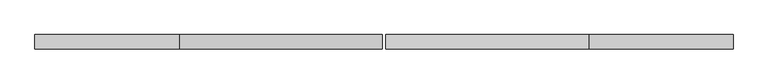
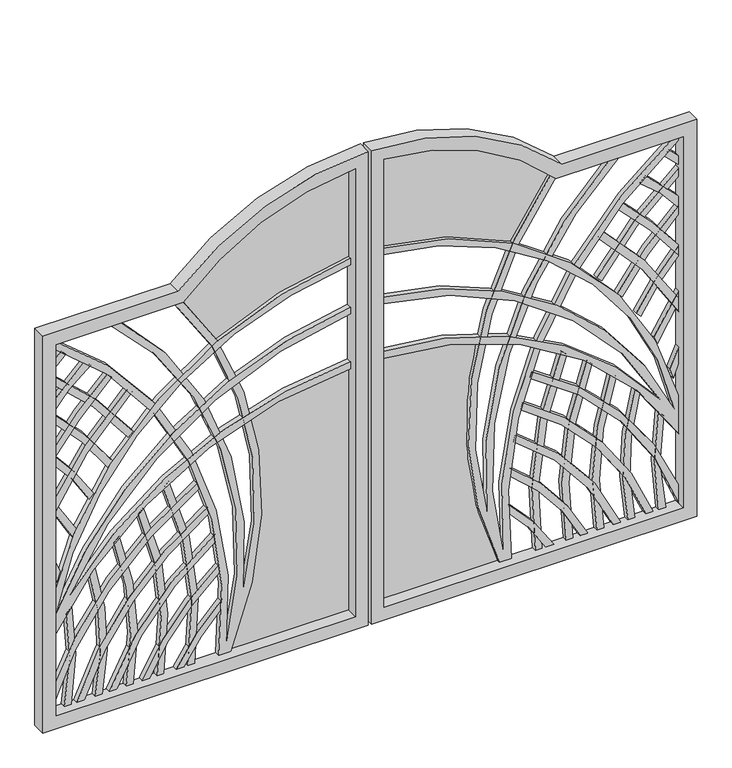
"""IFC4 building model written with IfcOpenShell, lengths in millimetres: proxy geometry."""

from ifc_helpers import new_model, si_unit, point, frame, frame_2d, origin, place, context, project, spatial, polyline, circle_curve, trimmed, segment, composite_curve, outline, extrude, source, transform, mapped, element, save


def generic_models_6bc30956(model_context):
    return source(origin(), model_context, "Body", "SweptSolid", [
        extrude(outline(composite_curve([segment(polyline([(1574.8, -714.375), (1574.8, -1222.375), (0.0, -1222.375), (0.0, 0.0), (1879.3736556, 0.0)]), True, "CONTINUOUS"), segment(trimmed(circle_curve(frame_2d((881.859553, 3.175)), 997.5191555), [point((1879.3736556, 0.0))], [point((1574.8, -714.375))], False, "CARTESIAN"), True, "CONTINUOUS")], self_intersect=False), holes=[composite_curve([segment(polyline([(1827.2147875, -47.625), (50.8, -47.625), (50.8, -1171.575), (1524.0, -1171.575), (1524.0, -692.4777911)]), True, "CONTINUOUS"), segment(trimmed(circle_curve(frame_2d((881.859553, 3.175)), 946.7191555), [point((1524.0, -692.4777911))], [point((1827.2147875, -47.625))], True, "CARTESIAN"), True, "CONTINUOUS")], self_intersect=False)]), frame((0.0, -50.8, 0.0), z_axis=(0.0, 1.0, 0.0), x_axis=(0.0, 0.0, 1.0)), (0.0, 0.0, 1.0), 50.8),
        extrude(outline(composite_curve([segment(trimmed(circle_curve(frame_2d((188.1193765, 65.6258097)), 1270.1981582), [point((1453.2587424, -47.625))], [point((475.7606767, -1171.575))], False, "CARTESIAN"), True, "CONTINUOUS"), segment(polyline([(475.7606767, -1171.575), (325.438753, -1171.575)]), True, "CONTINUOUS"), segment(trimmed(circle_curve(frame_2d((-306.470048, -9.2092819)), 1323.0278891), [point((325.438753, -1171.575))], [point((1016.0, -47.625))], True, "CARTESIAN"), True, "CONTINUOUS"), segment(polyline([(1016.0, -47.625), (1042.85139, -47.625)]), True, "CONTINUOUS"), segment(trimmed(circle_curve(frame_2d((-321.9912288, -1.7370637)), 1365.6138095), [point((1042.85139, -47.625))], [point((487.9033995, -1101.269586))], False, "CARTESIAN"), True, "CONTINUOUS"), segment(trimmed(circle_curve(frame_2d((-94.5667128, 101.7568292)), 1336.6166195), [point((487.9033995, -1101.269586))], [point((1233.6761327, -47.625))], True, "CARTESIAN"), True, "CONTINUOUS"), segment(polyline([(1233.6761327, -47.625), (1259.2332506, -47.625)]), True, "CONTINUOUS"), segment(trimmed(circle_curve(frame_2d((-94.5667128, 101.7568292)), 1362.0166195), [point((1259.2332506, -47.625))], [point((428.8390935, -1155.6753295))], False, "CARTESIAN"), True, "CONTINUOUS"), segment(trimmed(circle_curve(frame_2d((188.1193765, 65.6258097)), 1244.7981582), [point((428.8390935, -1155.6753295))], [point((1427.7550927, -47.625))], True, "CARTESIAN"), True, "CONTINUOUS"), segment(polyline([(1427.7550927, -47.625), (1453.2587424, -47.625)]), True, "CONTINUOUS")], self_intersect=False)), frame((0.0, -19.05, 0.0), z_axis=(0.0, 1.0, 0.0), x_axis=(0.0, 0.0, 1.0)), (0.0, 0.0, 1.0), 19.05),
        extrude(outline(composite_curve([segment(trimmed(circle_curve(frame_2d((625.1927136, -1831.8247988)), 1451.1947292), [point((50.8, -499.1436094))], [point((1524.0, -692.4777911))], False, "CARTESIAN"), True, "CONTINUOUS"), segment(polyline([(1524.0, -692.4777911), (1524.0, -717.8616311), (1508.2761961, -712.4096154)]), True, "CONTINUOUS"), segment(trimmed(circle_curve(frame_2d((625.2005352, -1831.8604357)), 1425.8305516), [point((1508.2761961, -712.4096154))], [point((270.5135839, -450.849962))], True, "CARTESIAN"), True, "CONTINUOUS"), segment(trimmed(circle_curve(frame_2d((428.9211986, -1911.4736244)), 1469.1883662), [point((270.5135839, -450.849962))], [point((1524.0, -932.0263955))], False, "CARTESIAN"), True, "CONTINUOUS"), segment(polyline([(1524.0, -932.0263955), (1524.0, -970.5462776)]), True, "CONTINUOUS"), segment(trimmed(circle_curve(frame_2d((434.6192112, -1905.6521568)), 1435.6787622), [point((1524.0, -970.5462776))], [point((79.5169904, -514.5820935))], True, "CARTESIAN"), True, "CONTINUOUS"), segment(trimmed(circle_curve(frame_2d((251.9754674, -2051.8469137)), 1546.9082241), [point((79.5169904, -514.5820935))], [point((1524.0, -1171.575))], False, "CARTESIAN"), True, "CONTINUOUS"), segment(polyline([(1524.0, -1171.575), (1492.986601, -1171.575)]), True, "CONTINUOUS"), segment(trimmed(circle_curve(frame_2d((251.9754674, -2051.8469137)), 1521.5082241), [point((1492.986601, -1171.575))], [point((50.8, -543.6971508))], True, "CARTESIAN"), True, "CONTINUOUS"), segment(polyline([(50.8, -543.6971508), (50.8, -499.1436094)]), True, "CONTINUOUS")], self_intersect=False)), frame((0.0, -19.05, 0.0), z_axis=(0.0, 1.0, 0.0), x_axis=(0.0, 0.0, 1.0)), (0.0, 0.0, 1.0), 19.05),
        extrude(outline(composite_curve([segment(trimmed(circle_curve(frame_2d((-321.9912288, -1.7370636)), 1251.3138095), [point((766.023996, -619.8059275))], [point((122.1545272, -1171.575))], False, "CARTESIAN"), True, "CONTINUOUS"), segment(polyline([(122.1545272, -1171.575), (50.8, -1171.575)]), True, "CONTINUOUS"), segment(trimmed(circle_curve(frame_2d((-329.3476454, 3.2021804)), 1234.7524675), [point((50.8, -1171.575))], [point((741.6413557, -611.2864))], True, "CARTESIAN"), True, "CONTINUOUS"), segment(polyline([(741.6413557, -611.2864), (766.023996, -619.8059275)]), True, "CONTINUOUS")], self_intersect=False)), frame((0.0, -19.05, 0.0), z_axis=(0.0, 1.0, 0.0), x_axis=(0.0, 0.0, 1.0)), (0.0, 0.0, 1.0), 19.05),
        extrude(outline(composite_curve([segment(trimmed(circle_curve(frame_2d((-321.9912288, -1.7370637)), 1137.0138095), [point((654.3216834, -584.5007383))], [point((50.8, -1075.9005069))], False, "CARTESIAN"), True, "CONTINUOUS"), segment(polyline([(50.8, -1075.9005069), (50.8, -1048.9772277)]), True, "CONTINUOUS"), segment(trimmed(circle_curve(frame_2d((-321.9912288, -1.7370637)), 1111.6138095), [point((50.8, -1048.9772277))], [point((628.7552213, -577.7287729))], True, "CARTESIAN"), True, "CONTINUOUS"), segment(polyline([(628.7552213, -577.7287729), (654.3216834, -584.5007383)]), True, "CONTINUOUS")], self_intersect=False)), frame((0.0, -19.05, 0.0), z_axis=(0.0, 1.0, 0.0), x_axis=(0.0, 0.0, 1.0)), (0.0, 0.0, 1.0), 19.05),
        extrude(outline(composite_curve([segment(trimmed(circle_curve(frame_2d((-321.9912288, -1.7370637)), 1022.7138095), [point((536.7182406, -557.2202617))], [point((50.8, -954.0869132))], False, "CARTESIAN"), True, "CONTINUOUS"), segment(polyline([(50.8, -954.0869132), (50.8, -926.7568118)]), True, "CONTINUOUS"), segment(trimmed(circle_curve(frame_2d((-321.9912288, -1.7370637)), 997.3138095), [point((50.8, -926.7568118))], [point((510.8571668, -550.3702604))], True, "CARTESIAN"), True, "CONTINUOUS"), segment(polyline([(510.8571668, -550.3702604), (536.7182406, -557.2202617)]), True, "CONTINUOUS")], self_intersect=False)), frame((0.0, -19.05, 0.0), z_axis=(0.0, 1.0, 0.0), x_axis=(0.0, 0.0, 1.0)), (0.0, 0.0, 1.0), 19.05),
        extrude(outline(composite_curve([segment(trimmed(circle_curve(frame_2d((-321.9912288, -1.7370637)), 908.4138095), [point((410.7722159, -538.6480277))], [point((50.8, -830.134522))], False, "CARTESIAN"), True, "CONTINUOUS"), segment(polyline([(50.8, -830.134522), (50.8, -802.1994847)]), True, "CONTINUOUS"), segment(trimmed(circle_curve(frame_2d((-321.9912288, -1.7370637)), 883.0138095), [point((50.8, -802.1994847))], [point((379.0365912, -538.6480277))], True, "CARTESIAN"), True, "CONTINUOUS"), segment(polyline([(379.0365912, -538.6480277), (410.7722159, -538.6480277)]), True, "CONTINUOUS")], self_intersect=False)), frame((0.0, -19.05, 0.0), z_axis=(0.0, 1.0, 0.0), x_axis=(0.0, 0.0, 1.0)), (0.0, 0.0, 1.0), 19.05),
        extrude(outline(composite_curve([segment(trimmed(circle_curve(frame_2d((-321.9912288, -1.7370637)), 794.1138095), [point((270.5266887, -530.4517881))], [point((50.8, -702.9099683))], False, "CARTESIAN"), True, "CONTINUOUS"), segment(polyline([(50.8, -702.9099683), (50.8, -674.0075603)]), True, "CONTINUOUS"), segment(trimmed(circle_curve(frame_2d((-321.9912288, -1.7370637)), 768.7138095), [point((50.8, -674.0075603))], [point((236.0245963, -530.4517881))], True, "CARTESIAN"), True, "CONTINUOUS"), segment(polyline([(236.0245963, -530.4517881), (270.5266887, -530.4517881)]), True, "CONTINUOUS")], self_intersect=False)), frame((0.0, -19.05, 0.0), z_axis=(0.0, 1.0, 0.0), x_axis=(0.0, 0.0, 1.0)), (0.0, 0.0, 1.0), 19.05),
        extrude(outline(composite_curve([segment(polyline([(1210.9602193, -867.4506933), (1228.939295, -885.429769)]), True, "CONTINUOUS"), segment(trimmed(circle_curve(frame_2d((188.1193765, 65.6258097)), 1409.8981582), [point((1228.939295, -885.429769))], [point((864.245824, -1171.575))], False, "CARTESIAN"), True, "CONTINUOUS"), segment(polyline([(864.245824, -1171.575), (809.5445985, -1171.575)]), True, "CONTINUOUS"), segment(trimmed(circle_curve(frame_2d((188.1193765, 65.6258097)), 1384.4981582), [point((809.5445985, -1171.575))], [point((1210.9602193, -867.4506933))], True, "CARTESIAN"), True, "CONTINUOUS")], self_intersect=False)), frame((0.0, -19.05, 0.0), z_axis=(0.0, 1.0, 0.0), x_axis=(0.0, 0.0, 1.0)), (0.0, 0.0, 1.0), 19.05),
        extrude(outline(composite_curve([segment(polyline([(1295.7670706, -944.0833092), (1313.7464656, -962.0627043)]), True, "CONTINUOUS"), segment(trimmed(circle_curve(frame_2d((298.9547736, -40.580869)), 1370.7410225), [point((1313.7464656, -962.0627043))], [point((1073.4115036, -1171.575))], False, "CARTESIAN"), True, "CONTINUOUS"), segment(polyline([(1073.4115036, -1171.575), (1034.1276953, -1171.575)]), True, "CONTINUOUS"), segment(trimmed(circle_curve(frame_2d((188.1193765, 65.6258097)), 1498.7981582), [point((1034.1276953, -1171.575))], [point((1295.7670706, -944.0833092))], True, "CARTESIAN"), True, "CONTINUOUS")], self_intersect=False)), frame((0.0, -19.05, 0.0), z_axis=(0.0, 1.0, 0.0), x_axis=(0.0, 0.0, 1.0)), (0.0, 0.0, 1.0), 19.05),
        extrude(outline(composite_curve([segment(polyline([(1371.3808408, -1023.8325474), (1393.8084123, -1046.2601189)]), True, "CONTINUOUS"), segment(trimmed(circle_curve(frame_2d((157.0059526, 65.2274597)), 1662.854462), [point((1393.8084123, -1046.2601189))], [point((1268.4935312, -1171.575))], False, "CARTESIAN"), True, "CONTINUOUS"), segment(polyline([(1268.4935312, -1171.575), (1223.2134903, -1171.575)]), True, "CONTINUOUS"), segment(trimmed(circle_curve(frame_2d((881.0604584, -680.2699964)), 598.7063586), [point((1223.2134903, -1171.575))], [point((1371.3808408, -1023.8325474))], True, "CARTESIAN"), True, "CONTINUOUS")], self_intersect=False)), frame((0.0, -19.05, 0.0), z_axis=(0.0, 1.0, 0.0), x_axis=(0.0, 0.0, 1.0)), (0.0, 0.0, 1.0), 19.05),
        extrude(outline(composite_curve([segment(polyline([(1448.1437026, -1116.942791), (1466.2607278, -1135.0598162)]), True, "CONTINUOUS"), segment(trimmed(circle_curve(frame_2d((2369.5144168, -2074.828689)), 1303.469509), [point((1466.2607278, -1135.0598162))], [point((1429.745544, -1171.575))], True, "CARTESIAN"), True, "CONTINUOUS"), segment(polyline([(1429.745544, -1171.575), (1393.6228205, -1171.575)]), True, "CONTINUOUS"), segment(trimmed(circle_curve(frame_2d((2581.8039176, -2302.8138821)), 1640.5717686), [point((1393.6228205, -1171.575))], [point((1448.1437026, -1116.942791))], False, "CARTESIAN"), True, "CONTINUOUS")], self_intersect=False)), frame((0.0, -19.05, 0.0), z_axis=(0.0, 1.0, 0.0), x_axis=(0.0, 0.0, 1.0)), (0.0, 0.0, 1.0), 19.05),
        extrude(outline(composite_curve([segment(polyline([(50.8, -1123.3836365), (50.8, -1096.2682984)]), True, "CONTINUOUS"), segment(trimmed(circle_curve(frame_2d((249.227799, -2294.693819)), 1214.741668), [point((50.8, -1096.2682984))], [point((439.2593722, -1094.9082877))], False, "CARTESIAN"), True, "CONTINUOUS"), segment(polyline([(439.2593722, -1094.9082877), (417.7529701, -1116.4146899)]), True, "CONTINUOUS"), segment(trimmed(circle_curve(frame_2d((251.9754674, -2051.8469137)), 950.0082241), [point((417.7529701, -1116.4146899))], [point((50.8, -1123.3836365))], True, "CARTESIAN"), True, "CONTINUOUS")], self_intersect=False)), frame((0.0, -19.05, 0.0), z_axis=(0.0, 1.0, 0.0), x_axis=(0.0, 0.0, 1.0)), (0.0, 0.0, 1.0), 19.05),
        extrude(outline(composite_curve([segment(polyline([(50.8, -1006.7247069), (50.8, -980.869582)]), True, "CONTINUOUS"), segment(trimmed(circle_curve(frame_2d((251.9754674, -2051.8469137)), 1089.7082241), [point((50.8, -980.869582))], [point((559.4182819, -1006.4078053))], False, "CARTESIAN"), True, "CONTINUOUS"), segment(polyline([(559.4182819, -1006.4078053), (538.8861292, -1026.939958)]), True, "CONTINUOUS"), segment(trimmed(circle_curve(frame_2d((251.9754674, -2051.8469137)), 1064.3082241), [point((538.8861292, -1026.939958))], [point((50.8, -1006.7247069))], True, "CARTESIAN"), True, "CONTINUOUS")], self_intersect=False)), frame((0.0, -19.05, 0.0), z_axis=(0.0, 1.0, 0.0), x_axis=(0.0, 0.0, 1.0)), (0.0, 0.0, 1.0), 19.05),
        extrude(outline(composite_curve([segment(polyline([(50.8, -890.30598), (50.8, -864.7646777)]), True, "CONTINUOUS"), segment(trimmed(circle_curve(frame_2d((251.9754674, -2051.8469137)), 1204.0082241), [point((50.8, -864.7646777))], [point((656.0575932, -917.6716895))], False, "CARTESIAN"), True, "CONTINUOUS"), segment(polyline([(656.0575932, -917.6716895), (636.1282841, -937.6009986)]), True, "CONTINUOUS"), segment(trimmed(circle_curve(frame_2d((249.671635, -2074.7397377)), 1201.0134277), [point((636.1282841, -937.6009986))], [point((50.8, -890.30598))], True, "CARTESIAN"), True, "CONTINUOUS")], self_intersect=False)), frame((0.0, -19.05, 0.0), z_axis=(0.0, 1.0, 0.0), x_axis=(0.0, 0.0, 1.0)), (0.0, 0.0, 1.0), 19.05),
        extrude(outline(composite_curve([segment(polyline([(50.8, -774.6859578), (50.8, -748.9789216)]), True, "CONTINUOUS"), segment(trimmed(circle_curve(frame_2d((251.9754674, -2051.8469137)), 1318.3082241), [point((50.8, -748.9789216))], [point((737.9350335, -826.3756274))], False, "CARTESIAN"), True, "CONTINUOUS"), segment(polyline([(737.9350335, -826.3756274), (718.3335001, -845.9771607)]), True, "CONTINUOUS"), segment(trimmed(circle_curve(frame_2d((251.9754674, -2051.8469137)), 1292.9082241), [point((718.3335001, -845.9771607))], [point((50.8, -774.6859578))], True, "CARTESIAN"), True, "CONTINUOUS")], self_intersect=False)), frame((0.0, -19.05, 0.0), z_axis=(0.0, 1.0, 0.0), x_axis=(0.0, 0.0, 1.0)), (0.0, 0.0, 1.0), 19.05),
        extrude(outline(composite_curve([segment(polyline([(50.8, -659.0930168), (50.8, -633.4341547)]), True, "CONTINUOUS"), segment(trimmed(circle_curve(frame_2d((251.9754674, -2051.8469137)), 1432.6082241), [point((50.8, -633.4341547))], [point((808.380048, -731.7028813))], False, "CARTESIAN"), True, "CONTINUOUS"), segment(polyline([(808.380048, -731.7028813), (788.9599222, -751.1230071)]), True, "CONTINUOUS"), segment(trimmed(circle_curve(frame_2d((251.9754674, -2051.8469137)), 1407.2082241), [point((788.9599222, -751.1230071))], [point((50.8, -659.0930168))], True, "CARTESIAN"), True, "CONTINUOUS")], self_intersect=False)), frame((0.0, -19.05, 0.0), z_axis=(0.0, 1.0, 0.0), x_axis=(0.0, 0.0, 1.0)), (0.0, 0.0, 1.0), 19.05),
        extrude(outline(polyline([(553.3842288, -1150.9205103), (593.450224, -1138.1641492), (672.1451492, -1171.575), (609.2386529, -1171.575), (553.3842288, -1150.9205103)])), frame((0.0, -19.05, 0.0), z_axis=(0.0, 1.0, 0.0), x_axis=(0.0, 0.0, 1.0)), (0.0, 0.0, 1.0), 19.05),
        extrude(outline(composite_curve([segment(trimmed(circle_curve(frame_2d((251.9754673, -2051.8469137)), 1064.3082241), [point((850.2006371, -1171.575))], [point((711.3700205, -1091.7903318))], True, "CARTESIAN"), True, "CONTINUOUS"), segment(polyline([(711.3700205, -1091.7903318), (740.9012216, -1077.980588)]), True, "CONTINUOUS"), segment(trimmed(circle_curve(frame_2d((251.9754674, -2051.8469137)), 1089.7082241), [point((740.9012216, -1077.980588))], [point((894.3035545, -1171.575))], False, "CARTESIAN"), True, "CONTINUOUS"), segment(polyline([(894.3035545, -1171.575), (850.2006371, -1171.575)]), True, "CONTINUOUS")], self_intersect=False)), frame((0.0, -19.05, 0.0), z_axis=(0.0, 1.0, 0.0), x_axis=(0.0, 0.0, 1.0)), (0.0, 0.0, 1.0), 19.05),
        extrude(outline(composite_curve([segment(trimmed(circle_curve(frame_2d((436.5150762, -1780.3292563)), 853.0665783), [point((1034.1276953, -1171.575))], [point((842.2813497, -1029.9451424))], True, "CARTESIAN"), True, "CONTINUOUS"), segment(polyline([(842.2813497, -1029.9451424), (859.7363544, -1012.4901377)]), True, "CONTINUOUS"), segment(trimmed(circle_curve(frame_2d((251.9754673, -2051.8469137)), 1204.0082241), [point((859.7363544, -1012.4901377))], [point((1073.4115036, -1171.575))], False, "CARTESIAN"), True, "CONTINUOUS"), segment(polyline([(1073.4115036, -1171.575), (1034.1276953, -1171.575)]), True, "CONTINUOUS")], self_intersect=False)), frame((0.0, -19.05, 0.0), z_axis=(0.0, 1.0, 0.0), x_axis=(0.0, 0.0, 1.0)), (0.0, 0.0, 1.0), 19.05),
        extrude(outline(composite_curve([segment(polyline([(943.9740273, -959.7161207), (962.3717805, -941.3183675)]), True, "CONTINUOUS"), segment(trimmed(circle_curve(frame_2d((251.9754673, -2051.8469138)), 1318.3082242), [point((962.3717805, -941.3183675))], [point((1233.3306179, -1171.575))], False, "CARTESIAN"), True, "CONTINUOUS"), segment(polyline([(1233.3306179, -1171.575), (1198.9353576, -1171.575)]), True, "CONTINUOUS"), segment(trimmed(circle_curve(frame_2d((251.9754673, -2051.8469138)), 1292.9082241), [point((1198.9353576, -1171.575))], [point((943.9740273, -959.7161207))], True, "CARTESIAN"), True, "CONTINUOUS")], self_intersect=False)), frame((0.0, -19.05, 0.0), z_axis=(0.0, 1.0, 0.0), x_axis=(0.0, 0.0, 1.0)), (0.0, 0.0, 1.0), 19.05),
        extrude(outline(composite_curve([segment(polyline([(1035.0267606, -882.6310833), (1053.3289179, -864.3289261)]), True, "CONTINUOUS"), segment(trimmed(circle_curve(frame_2d((251.9754673, -2051.8469137)), 1432.6082241), [point((1053.3289179, -864.3289261))], [point((1382.2354736, -1171.575))], False, "CARTESIAN"), True, "CONTINUOUS"), segment(polyline([(1382.2354736, -1171.575), (1349.8626855, -1171.575)]), True, "CONTINUOUS"), segment(trimmed(circle_curve(frame_2d((251.9754674, -2051.8469137)), 1407.2082241), [point((1349.8626855, -1171.575))], [point((1035.0267606, -882.6310833))], True, "CARTESIAN"), True, "CONTINUOUS")], self_intersect=False)), frame((0.0, -19.05, 0.0), z_axis=(0.0, 1.0, 0.0), x_axis=(0.0, 0.0, 1.0)), (0.0, 0.0, 1.0), 19.05),
        extrude(outline(composite_curve([segment(trimmed(circle_curve(frame_2d((881.859553, 3.175)), 946.7191555), [point((1827.2147875, -47.625))], [point((1524.0, -692.4777911))], False, "CARTESIAN"), True, "CONTINUOUS"), segment(trimmed(circle_curve(frame_2d((625.1927137, -1831.8247988)), 1451.1947292), [point((1524.0, -692.4777911))], [point((1300.6036994, -547.3847876))], True, "CARTESIAN"), True, "CONTINUOUS"), segment(trimmed(circle_curve(frame_2d((188.1193765, 65.6258097)), 1270.1981582), [point((1300.6036994, -547.3847876))], [point((1453.2587424, -47.625))], True, "CARTESIAN"), True, "CONTINUOUS"), segment(polyline([(1453.2587424, -47.625), (1827.2147875, -47.625)]), True, "CONTINUOUS")], self_intersect=False)), frame((0.0, -6.35, 0.0), z_axis=(0.0, 1.0, 0.0), x_axis=(0.0, 0.0, 1.0)), (0.0, 0.0, 1.0), 6.35),
        extrude(outline(composite_curve([segment(trimmed(circle_curve(frame_2d((-306.470048, -9.2092819)), 1323.0278891), [point((1016.0, -47.625))], [point((951.8602911, -417.8748577))], False, "CARTESIAN"), True, "CONTINUOUS"), segment(trimmed(circle_curve(frame_2d((625.1927136, -1831.8247988)), 1451.1947292), [point((951.8602911, -417.8748577))], [point((50.8, -499.1436094))], True, "CARTESIAN"), True, "CONTINUOUS"), segment(polyline([(50.8, -499.1436094), (50.8, -47.625), (1016.0, -47.625)]), True, "CONTINUOUS")], self_intersect=False)), frame((0.0, -6.35, 0.0), z_axis=(0.0, 1.0, 0.0), x_axis=(0.0, 0.0, 1.0)), (0.0, 0.0, 1.0), 6.35),
        extrude(outline(composite_curve([segment(trimmed(circle_curve(frame_2d((881.859553, 9.525)), 997.5191555), [point((1574.8, 727.075))], [point((1879.3736556, 12.7))], False, "CARTESIAN"), True, "CONTINUOUS"), segment(polyline([(1879.3736556, 12.7), (0.0, 12.7), (0.0, 1235.075), (1574.8, 1235.075), (1574.8, 727.075)]), True, "CONTINUOUS")], self_intersect=False), holes=[composite_curve([segment(trimmed(circle_curve(frame_2d((881.859553, 9.525)), 946.7191555), [point((1827.2147875, 60.325))], [point((1524.0, 705.1777911))], True, "CARTESIAN"), True, "CONTINUOUS"), segment(polyline([(1524.0, 705.1777911), (1524.0, 1184.275), (50.8, 1184.275), (50.8, 60.325), (1827.2147875, 60.325)]), True, "CONTINUOUS")], self_intersect=False)]), frame((0.0, -50.8, 0.0), z_axis=(0.0, 1.0, 0.0), x_axis=(0.0, 0.0, 1.0)), (0.0, 0.0, 1.0), 50.8),
        extrude(outline(composite_curve([segment(polyline([(1453.2587424, 60.325), (1427.7550927, 60.325)]), True, "CONTINUOUS"), segment(trimmed(circle_curve(frame_2d((188.1193765, -52.9258097)), 1244.7981582), [point((1427.7550927, 60.325))], [point((428.8390935, 1168.3753295))], True, "CARTESIAN"), True, "CONTINUOUS"), segment(trimmed(circle_curve(frame_2d((-94.5667128, -89.0568292)), 1362.0166195), [point((428.8390935, 1168.3753295))], [point((1259.2332506, 60.325))], False, "CARTESIAN"), True, "CONTINUOUS"), segment(polyline([(1259.2332506, 60.325), (1233.6761327, 60.325)]), True, "CONTINUOUS"), segment(trimmed(circle_curve(frame_2d((-94.5667128, -89.0568292)), 1336.6166195), [point((1233.6761327, 60.325))], [point((487.9033995, 1113.969586))], True, "CARTESIAN"), True, "CONTINUOUS"), segment(trimmed(circle_curve(frame_2d((-321.9912288, 14.4370637)), 1365.6138095), [point((487.9033995, 1113.969586))], [point((1042.85139, 60.325))], False, "CARTESIAN"), True, "CONTINUOUS"), segment(polyline([(1042.85139, 60.325), (1016.0, 60.325)]), True, "CONTINUOUS"), segment(trimmed(circle_curve(frame_2d((-306.470048, 21.9092819)), 1323.0278891), [point((1016.0, 60.325))], [point((325.438753, 1184.275))], True, "CARTESIAN"), True, "CONTINUOUS"), segment(polyline([(325.438753, 1184.275), (475.7606767, 1184.275)]), True, "CONTINUOUS"), segment(trimmed(circle_curve(frame_2d((188.1193765, -52.9258097)), 1270.1981582), [point((475.7606767, 1184.275))], [point((1453.2587424, 60.325))], False, "CARTESIAN"), True, "CONTINUOUS")], self_intersect=False)), frame((0.0, -19.05, 0.0), z_axis=(0.0, 1.0, 0.0), x_axis=(0.0, 0.0, 1.0)), (0.0, 0.0, 1.0), 19.05),
        extrude(outline(composite_curve([segment(polyline([(50.8, 511.8436094), (50.8, 556.3971508)]), True, "CONTINUOUS"), segment(trimmed(circle_curve(frame_2d((251.9754674, 2064.5469137)), 1521.5082241), [point((50.8, 556.3971508))], [point((1492.986601, 1184.275))], True, "CARTESIAN"), True, "CONTINUOUS"), segment(polyline([(1492.986601, 1184.275), (1524.0, 1184.275)]), True, "CONTINUOUS"), segment(trimmed(circle_curve(frame_2d((251.9754674, 2064.5469137)), 1546.9082241), [point((1524.0, 1184.275))], [point((79.5169904, 527.2820935))], False, "CARTESIAN"), True, "CONTINUOUS"), segment(trimmed(circle_curve(frame_2d((434.6192112, 1918.3521568)), 1435.6787622), [point((79.5169904, 527.2820935))], [point((1524.0, 983.2462776))], True, "CARTESIAN"), True, "CONTINUOUS"), segment(polyline([(1524.0, 983.2462776), (1524.0, 944.7263955)]), True, "CONTINUOUS"), segment(trimmed(circle_curve(frame_2d((428.9211986, 1924.1736244)), 1469.1883662), [point((1524.0, 944.7263955))], [point((270.5135839, 463.549962))], False, "CARTESIAN"), True, "CONTINUOUS"), segment(trimmed(circle_curve(frame_2d((625.2005352, 1844.5604357)), 1425.8305516), [point((270.5135839, 463.549962))], [point((1508.2761961, 725.1096154))], True, "CARTESIAN"), True, "CONTINUOUS"), segment(polyline([(1508.2761961, 725.1096154), (1524.0, 730.5616311), (1524.0, 705.1777911)]), True, "CONTINUOUS"), segment(trimmed(circle_curve(frame_2d((625.1927136, 1844.5247988)), 1451.1947292), [point((1524.0, 705.1777911))], [point((50.8, 511.8436094))], False, "CARTESIAN"), True, "CONTINUOUS")], self_intersect=False)), frame((0.0, -19.05, 0.0), z_axis=(0.0, 1.0, 0.0), x_axis=(0.0, 0.0, 1.0)), (0.0, 0.0, 1.0), 19.05),
        extrude(outline(composite_curve([segment(polyline([(766.023996, 632.5059275), (741.6413557, 623.9864)]), True, "CONTINUOUS"), segment(trimmed(circle_curve(frame_2d((-329.3476454, 9.4978196)), 1234.7524675), [point((741.6413557, 623.9864))], [point((50.8, 1184.275))], True, "CARTESIAN"), True, "CONTINUOUS"), segment(polyline([(50.8, 1184.275), (122.1545272, 1184.275)]), True, "CONTINUOUS"), segment(trimmed(circle_curve(frame_2d((-321.9912288, 14.4370636)), 1251.3138095), [point((122.1545272, 1184.275))], [point((766.023996, 632.5059275))], False, "CARTESIAN"), True, "CONTINUOUS")], self_intersect=False)), frame((0.0, -19.05, 0.0), z_axis=(0.0, 1.0, 0.0), x_axis=(0.0, 0.0, 1.0)), (0.0, 0.0, 1.0), 19.05),
        extrude(outline(composite_curve([segment(polyline([(654.3216834, 597.2007383), (628.7552213, 590.4287729)]), True, "CONTINUOUS"), segment(trimmed(circle_curve(frame_2d((-321.9912288, 14.4370637)), 1111.6138095), [point((628.7552213, 590.4287729))], [point((50.8, 1061.6772277))], True, "CARTESIAN"), True, "CONTINUOUS"), segment(polyline([(50.8, 1061.6772277), (50.8, 1088.6005069)]), True, "CONTINUOUS"), segment(trimmed(circle_curve(frame_2d((-321.9912288, 14.4370637)), 1137.0138095), [point((50.8, 1088.6005069))], [point((654.3216834, 597.2007383))], False, "CARTESIAN"), True, "CONTINUOUS")], self_intersect=False)), frame((0.0, -19.05, 0.0), z_axis=(0.0, 1.0, 0.0), x_axis=(0.0, 0.0, 1.0)), (0.0, 0.0, 1.0), 19.05),
        extrude(outline(composite_curve([segment(polyline([(536.7182406, 569.9202617), (510.8571668, 563.0702604)]), True, "CONTINUOUS"), segment(trimmed(circle_curve(frame_2d((-321.9912288, 14.4370637)), 997.3138095), [point((510.8571668, 563.0702604))], [point((50.8, 939.4568118))], True, "CARTESIAN"), True, "CONTINUOUS"), segment(polyline([(50.8, 939.4568118), (50.8, 966.7869132)]), True, "CONTINUOUS"), segment(trimmed(circle_curve(frame_2d((-321.9912288, 14.4370637)), 1022.7138095), [point((50.8, 966.7869132))], [point((536.7182406, 569.9202617))], False, "CARTESIAN"), True, "CONTINUOUS")], self_intersect=False)), frame((0.0, -19.05, 0.0), z_axis=(0.0, 1.0, 0.0), x_axis=(0.0, 0.0, 1.0)), (0.0, 0.0, 1.0), 19.05),
        extrude(outline(composite_curve([segment(polyline([(410.7722159, 551.3480277), (379.0365912, 551.3480277)]), True, "CONTINUOUS"), segment(trimmed(circle_curve(frame_2d((-321.9912288, 14.4370637)), 883.0138095), [point((379.0365912, 551.3480277))], [point((50.8, 814.8994847))], True, "CARTESIAN"), True, "CONTINUOUS"), segment(polyline([(50.8, 814.8994847), (50.8, 842.834522)]), True, "CONTINUOUS"), segment(trimmed(circle_curve(frame_2d((-321.9912288, 14.4370637)), 908.4138095), [point((50.8, 842.834522))], [point((410.7722159, 551.3480277))], False, "CARTESIAN"), True, "CONTINUOUS")], self_intersect=False)), frame((0.0, -19.05, 0.0), z_axis=(0.0, 1.0, 0.0), x_axis=(0.0, 0.0, 1.0)), (0.0, 0.0, 1.0), 19.05),
        extrude(outline(composite_curve([segment(polyline([(270.5266887, 543.1517881), (236.0245963, 543.1517881)]), True, "CONTINUOUS"), segment(trimmed(circle_curve(frame_2d((-321.9912288, 14.4370637)), 768.7138095), [point((236.0245963, 543.1517881))], [point((50.8, 686.7075603))], True, "CARTESIAN"), True, "CONTINUOUS"), segment(polyline([(50.8, 686.7075603), (50.8, 715.6099683)]), True, "CONTINUOUS"), segment(trimmed(circle_curve(frame_2d((-321.9912288, 14.4370637)), 794.1138095), [point((50.8, 715.6099683))], [point((270.5266887, 543.1517881))], False, "CARTESIAN"), True, "CONTINUOUS")], self_intersect=False)), frame((0.0, -19.05, 0.0), z_axis=(0.0, 1.0, 0.0), x_axis=(0.0, 0.0, 1.0)), (0.0, 0.0, 1.0), 19.05),
        extrude(outline(composite_curve([segment(trimmed(circle_curve(frame_2d((188.1193765, -52.9258097)), 1384.4981582), [point((1210.9602193, 880.1506933))], [point((809.5445985, 1184.275))], True, "CARTESIAN"), True, "CONTINUOUS"), segment(polyline([(809.5445985, 1184.275), (864.245824, 1184.275)]), True, "CONTINUOUS"), segment(trimmed(circle_curve(frame_2d((188.1193765, -52.9258097)), 1409.8981582), [point((864.245824, 1184.275))], [point((1228.939295, 898.129769))], False, "CARTESIAN"), True, "CONTINUOUS"), segment(polyline([(1228.939295, 898.129769), (1210.9602193, 880.1506933)]), True, "CONTINUOUS")], self_intersect=False)), frame((0.0, -19.05, 0.0), z_axis=(0.0, 1.0, 0.0), x_axis=(0.0, 0.0, 1.0)), (0.0, 0.0, 1.0), 19.05),
        extrude(outline(composite_curve([segment(trimmed(circle_curve(frame_2d((188.1193765, -52.9258097)), 1498.7981582), [point((1295.7670706, 956.7833092))], [point((1034.1276953, 1184.275))], True, "CARTESIAN"), True, "CONTINUOUS"), segment(polyline([(1034.1276953, 1184.275), (1073.4115036, 1184.275)]), True, "CONTINUOUS"), segment(trimmed(circle_curve(frame_2d((298.9547736, 53.280869)), 1370.7410225), [point((1073.4115036, 1184.275))], [point((1313.7464656, 974.7627043))], False, "CARTESIAN"), True, "CONTINUOUS"), segment(polyline([(1313.7464656, 974.7627043), (1295.7670706, 956.7833092)]), True, "CONTINUOUS")], self_intersect=False)), frame((0.0, -19.05, 0.0), z_axis=(0.0, 1.0, 0.0), x_axis=(0.0, 0.0, 1.0)), (0.0, 0.0, 1.0), 19.05),
        extrude(outline(composite_curve([segment(trimmed(circle_curve(frame_2d((881.0604584, 692.9699964)), 598.7063586), [point((1371.3808408, 1036.5325474))], [point((1223.2134903, 1184.275))], True, "CARTESIAN"), True, "CONTINUOUS"), segment(polyline([(1223.2134903, 1184.275), (1268.4935312, 1184.275)]), True, "CONTINUOUS"), segment(trimmed(circle_curve(frame_2d((157.0059526, -52.5274597)), 1662.854462), [point((1268.4935312, 1184.275))], [point((1393.8084123, 1058.9601189))], False, "CARTESIAN"), True, "CONTINUOUS"), segment(polyline([(1393.8084123, 1058.9601189), (1371.3808408, 1036.5325474)]), True, "CONTINUOUS")], self_intersect=False)), frame((0.0, -19.05, 0.0), z_axis=(0.0, 1.0, 0.0), x_axis=(0.0, 0.0, 1.0)), (0.0, 0.0, 1.0), 19.05),
        extrude(outline(composite_curve([segment(trimmed(circle_curve(frame_2d((2581.8039176, 2315.5138821)), 1640.5717686), [point((1448.1437026, 1129.642791))], [point((1393.6228205, 1184.275))], False, "CARTESIAN"), True, "CONTINUOUS"), segment(polyline([(1393.6228205, 1184.275), (1429.745544, 1184.275)]), True, "CONTINUOUS"), segment(trimmed(circle_curve(frame_2d((2369.5144168, 2087.528689)), 1303.469509), [point((1429.745544, 1184.275))], [point((1466.2607278, 1147.7598162))], True, "CARTESIAN"), True, "CONTINUOUS"), segment(polyline([(1466.2607278, 1147.7598162), (1448.1437026, 1129.642791)]), True, "CONTINUOUS")], self_intersect=False)), frame((0.0, -19.05, 0.0), z_axis=(0.0, 1.0, 0.0), x_axis=(0.0, 0.0, 1.0)), (0.0, 0.0, 1.0), 19.05),
        extrude(outline(composite_curve([segment(trimmed(circle_curve(frame_2d((251.9754674, 2064.5469137)), 950.0082241), [point((50.8, 1136.0836365))], [point((417.7529701, 1129.1146899))], True, "CARTESIAN"), True, "CONTINUOUS"), segment(polyline([(417.7529701, 1129.1146899), (439.2593722, 1107.6082877)]), True, "CONTINUOUS"), segment(trimmed(circle_curve(frame_2d((249.227799, 2307.393819)), 1214.741668), [point((439.2593722, 1107.6082877))], [point((50.8, 1108.9682984))], False, "CARTESIAN"), True, "CONTINUOUS"), segment(polyline([(50.8, 1108.9682984), (50.8, 1136.0836365)]), True, "CONTINUOUS")], self_intersect=False)), frame((0.0, -19.05, 0.0), z_axis=(0.0, 1.0, 0.0), x_axis=(0.0, 0.0, 1.0)), (0.0, 0.0, 1.0), 19.05),
        extrude(outline(composite_curve([segment(trimmed(circle_curve(frame_2d((251.9754674, 2064.5469137)), 1064.3082241), [point((50.8, 1019.4247069))], [point((538.8861292, 1039.639958))], True, "CARTESIAN"), True, "CONTINUOUS"), segment(polyline([(538.8861292, 1039.639958), (559.4182819, 1019.1078053)]), True, "CONTINUOUS"), segment(trimmed(circle_curve(frame_2d((251.9754674, 2064.5469137)), 1089.7082241), [point((559.4182819, 1019.1078053))], [point((50.8, 993.569582))], False, "CARTESIAN"), True, "CONTINUOUS"), segment(polyline([(50.8, 993.569582), (50.8, 1019.4247069)]), True, "CONTINUOUS")], self_intersect=False)), frame((0.0, -19.05, 0.0), z_axis=(0.0, 1.0, 0.0), x_axis=(0.0, 0.0, 1.0)), (0.0, 0.0, 1.0), 19.05),
        extrude(outline(composite_curve([segment(trimmed(circle_curve(frame_2d((249.671635, 2087.4397377)), 1201.0134277), [point((50.8, 903.00598))], [point((636.1282841, 950.3009986))], True, "CARTESIAN"), True, "CONTINUOUS"), segment(polyline([(636.1282841, 950.3009986), (656.0575932, 930.3716895)]), True, "CONTINUOUS"), segment(trimmed(circle_curve(frame_2d((251.9754674, 2064.5469137)), 1204.0082241), [point((656.0575932, 930.3716895))], [point((50.8, 877.4646777))], False, "CARTESIAN"), True, "CONTINUOUS"), segment(polyline([(50.8, 877.4646777), (50.8, 903.00598)]), True, "CONTINUOUS")], self_intersect=False)), frame((0.0, -19.05, 0.0), z_axis=(0.0, 1.0, 0.0), x_axis=(0.0, 0.0, 1.0)), (0.0, 0.0, 1.0), 19.05),
        extrude(outline(composite_curve([segment(trimmed(circle_curve(frame_2d((251.9754674, 2064.5469137)), 1292.9082241), [point((50.8, 787.3859578))], [point((718.3335001, 858.6771607))], True, "CARTESIAN"), True, "CONTINUOUS"), segment(polyline([(718.3335001, 858.6771607), (737.9350335, 839.0756274)]), True, "CONTINUOUS"), segment(trimmed(circle_curve(frame_2d((251.9754674, 2064.5469137)), 1318.3082241), [point((737.9350335, 839.0756274))], [point((50.8, 761.6789216))], False, "CARTESIAN"), True, "CONTINUOUS"), segment(polyline([(50.8, 761.6789216), (50.8, 787.3859578)]), True, "CONTINUOUS")], self_intersect=False)), frame((0.0, -19.05, 0.0), z_axis=(0.0, 1.0, 0.0), x_axis=(0.0, 0.0, 1.0)), (0.0, 0.0, 1.0), 19.05),
        extrude(outline(composite_curve([segment(trimmed(circle_curve(frame_2d((251.9754674, 2064.5469137)), 1407.2082241), [point((50.8, 671.7930168))], [point((788.9599222, 763.8230071))], True, "CARTESIAN"), True, "CONTINUOUS"), segment(polyline([(788.9599222, 763.8230071), (808.380048, 744.4028813)]), True, "CONTINUOUS"), segment(trimmed(circle_curve(frame_2d((251.9754674, 2064.5469137)), 1432.6082241), [point((808.380048, 744.4028813))], [point((50.8, 646.1341547))], False, "CARTESIAN"), True, "CONTINUOUS"), segment(polyline([(50.8, 646.1341547), (50.8, 671.7930168)]), True, "CONTINUOUS")], self_intersect=False)), frame((0.0, -19.05, 0.0), z_axis=(0.0, 1.0, 0.0), x_axis=(0.0, 0.0, 1.0)), (0.0, 0.0, 1.0), 19.05),
        extrude(outline(polyline([(553.3842288, 1163.6205103), (609.2386529, 1184.275), (672.1451492, 1184.275), (593.450224, 1150.8641492), (553.3842288, 1163.6205103)])), frame((0.0, -19.05, 0.0), z_axis=(0.0, 1.0, 0.0), x_axis=(0.0, 0.0, 1.0)), (0.0, 0.0, 1.0), 19.05),
        extrude(outline(composite_curve([segment(polyline([(850.2006371, 1184.275), (894.3035545, 1184.275)]), True, "CONTINUOUS"), segment(trimmed(circle_curve(frame_2d((251.9754674, 2064.5469137)), 1089.7082241), [point((894.3035545, 1184.275))], [point((740.9012216, 1090.680588))], False, "CARTESIAN"), True, "CONTINUOUS"), segment(polyline([(740.9012216, 1090.680588), (711.3700205, 1104.4903318)]), True, "CONTINUOUS"), segment(trimmed(circle_curve(frame_2d((251.9754673, 2064.5469137)), 1064.3082241), [point((711.3700205, 1104.4903318))], [point((850.2006371, 1184.275))], True, "CARTESIAN"), True, "CONTINUOUS")], self_intersect=False)), frame((0.0, -19.05, 0.0), z_axis=(0.0, 1.0, 0.0), x_axis=(0.0, 0.0, 1.0)), (0.0, 0.0, 1.0), 19.05),
        extrude(outline(composite_curve([segment(polyline([(1034.1276953, 1184.275), (1073.4115036, 1184.275)]), True, "CONTINUOUS"), segment(trimmed(circle_curve(frame_2d((251.9754673, 2064.5469137)), 1204.0082241), [point((1073.4115036, 1184.275))], [point((859.7363544, 1025.1901377))], False, "CARTESIAN"), True, "CONTINUOUS"), segment(polyline([(859.7363544, 1025.1901377), (842.2813497, 1042.6451424)]), True, "CONTINUOUS"), segment(trimmed(circle_curve(frame_2d((436.5150762, 1793.0292563)), 853.0665783), [point((842.2813497, 1042.6451424))], [point((1034.1276953, 1184.275))], True, "CARTESIAN"), True, "CONTINUOUS")], self_intersect=False)), frame((0.0, -19.05, 0.0), z_axis=(0.0, 1.0, 0.0), x_axis=(0.0, 0.0, 1.0)), (0.0, 0.0, 1.0), 19.05),
        extrude(outline(composite_curve([segment(trimmed(circle_curve(frame_2d((251.9754673, 2064.5469138)), 1292.9082241), [point((943.9740273, 972.4161207))], [point((1198.9353576, 1184.275))], True, "CARTESIAN"), True, "CONTINUOUS"), segment(polyline([(1198.9353576, 1184.275), (1233.3306179, 1184.275)]), True, "CONTINUOUS"), segment(trimmed(circle_curve(frame_2d((251.9754673, 2064.5469138)), 1318.3082242), [point((1233.3306179, 1184.275))], [point((962.3717805, 954.0183675))], False, "CARTESIAN"), True, "CONTINUOUS"), segment(polyline([(962.3717805, 954.0183675), (943.9740273, 972.4161207)]), True, "CONTINUOUS")], self_intersect=False)), frame((0.0, -19.05, 0.0), z_axis=(0.0, 1.0, 0.0), x_axis=(0.0, 0.0, 1.0)), (0.0, 0.0, 1.0), 19.05),
        extrude(outline(composite_curve([segment(trimmed(circle_curve(frame_2d((251.9754674, 2064.5469137)), 1407.2082241), [point((1035.0267606, 895.3310833))], [point((1349.8626855, 1184.275))], True, "CARTESIAN"), True, "CONTINUOUS"), segment(polyline([(1349.8626855, 1184.275), (1382.2354736, 1184.275)]), True, "CONTINUOUS"), segment(trimmed(circle_curve(frame_2d((251.9754673, 2064.5469137)), 1432.6082241), [point((1382.2354736, 1184.275))], [point((1053.3289179, 877.0289261))], False, "CARTESIAN"), True, "CONTINUOUS"), segment(polyline([(1053.3289179, 877.0289261), (1035.0267606, 895.3310833)]), True, "CONTINUOUS")], self_intersect=False)), frame((0.0, -19.05, 0.0), z_axis=(0.0, 1.0, 0.0), x_axis=(0.0, 0.0, 1.0)), (0.0, 0.0, 1.0), 19.05),
        extrude(outline(composite_curve([segment(polyline([(1827.2147875, 60.325), (1453.2587424, 60.325)]), True, "CONTINUOUS"), segment(trimmed(circle_curve(frame_2d((188.1193765, -52.9258097)), 1270.1981582), [point((1453.2587424, 60.325))], [point((1300.6036994, 560.0847876))], True, "CARTESIAN"), True, "CONTINUOUS"), segment(trimmed(circle_curve(frame_2d((625.1927137, 1844.5247988)), 1451.1947292), [point((1300.6036994, 560.0847876))], [point((1524.0, 705.1777911))], True, "CARTESIAN"), True, "CONTINUOUS"), segment(trimmed(circle_curve(frame_2d((881.859553, 9.525)), 946.7191555), [point((1524.0, 705.1777911))], [point((1827.2147875, 60.325))], False, "CARTESIAN"), True, "CONTINUOUS")], self_intersect=False)), frame((0.0, -6.35, 0.0), z_axis=(0.0, 1.0, 0.0), x_axis=(0.0, 0.0, 1.0)), (0.0, 0.0, 1.0), 6.35),
        extrude(outline(composite_curve([segment(polyline([(1016.0, 60.325), (50.8, 60.325), (50.8, 511.8436094)]), True, "CONTINUOUS"), segment(trimmed(circle_curve(frame_2d((625.1927136, 1844.5247988)), 1451.1947292), [point((50.8, 511.8436094))], [point((951.8602911, 430.5748577))], True, "CARTESIAN"), True, "CONTINUOUS"), segment(trimmed(circle_curve(frame_2d((-306.470048, 21.9092819)), 1323.0278891), [point((951.8602911, 430.5748577))], [point((1016.0, 60.325))], False, "CARTESIAN"), True, "CONTINUOUS")], self_intersect=False)), frame((0.0, -6.35, 0.0), z_axis=(0.0, 1.0, 0.0), x_axis=(0.0, 0.0, 1.0)), (0.0, 0.0, 1.0), 6.35),
    ])


if __name__ == "__main__":
    model = new_model("IFC4")
    model_context = context("Model", 3, world=origin())
    ifc_project = project(units=[si_unit("LENGTHUNIT", "METRE", prefix="MILLI")], contexts=[model_context])
    site = spatial("IfcSite", under=ifc_project)
    building = spatial("IfcBuilding", under=site)
    placement = place(None, origin())
    generic_models_shape = generic_models_6bc30956(model_context)
    element("IfcBuildingElementProxy", 1, Name="Generic Models", at=placement, inside=building, context=model_context, shape_type="MappedRepresentation", body=[
        mapped(generic_models_shape, transform((0.0, 0.0, 0.0), x_axis=(1.0, 0.0, 0.0), y_axis=(0.0, 1.0, 0.0), z_axis=(0.0, 0.0, 1.0))),
    ])
    save(model, "model.ifc")

# Revit data of these elements
# Type
#   m.s. sheet = none
#   2" x2" pipe = none
#   1"x1"pipe = none
#   Default Elevation = 0
# Element 1 (IfcBuildingElementProxy)
#   Materials on its faces: "r1"
# Materials
#   "r1": class "Generic", colour RGB 120 120 120, transparency 0, Cost = 0
